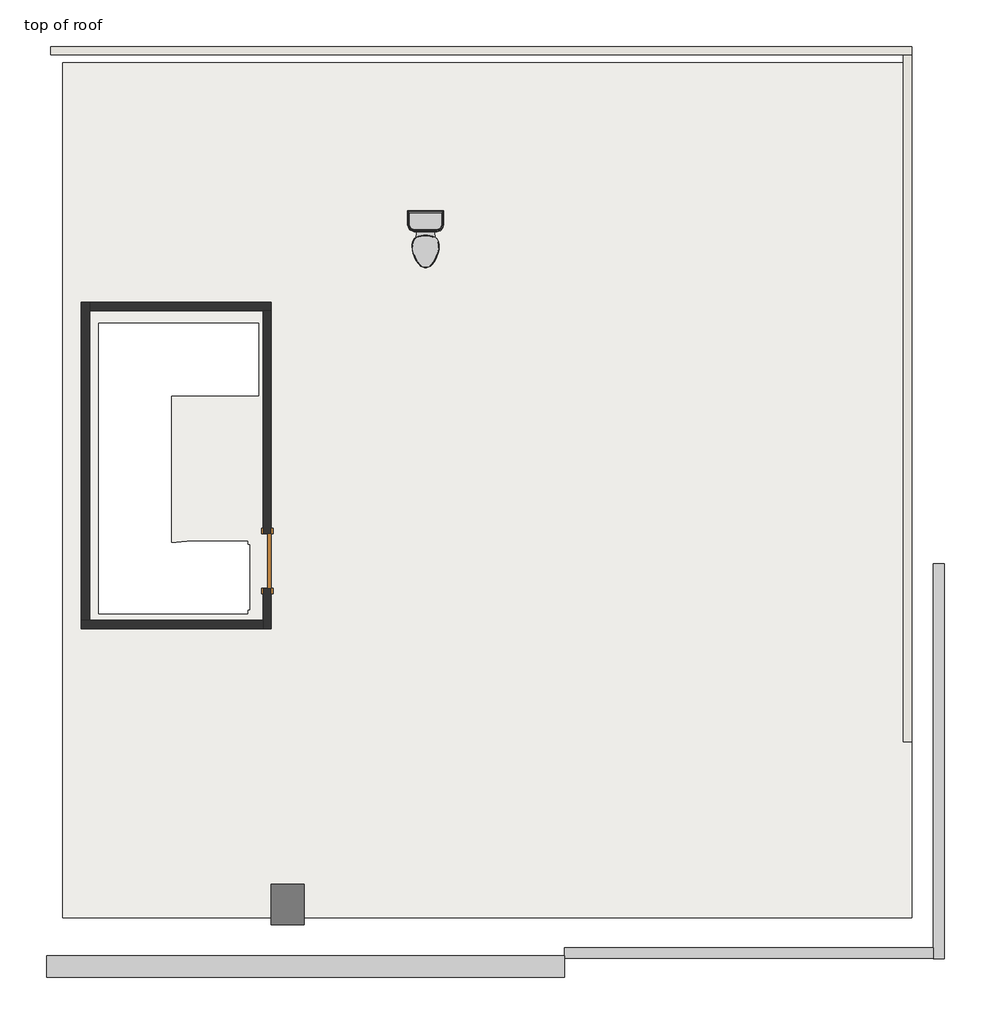
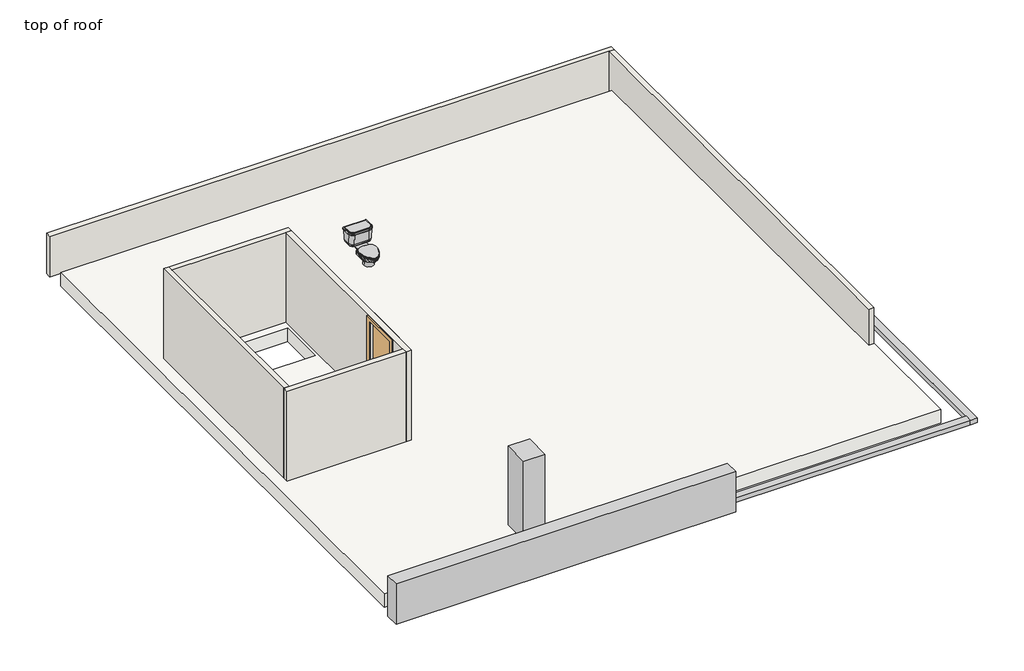
# One storey, incomplete: 6 walls, 4 proxies, 1 door, 1 flow terminal, 1 slab.
"""IFC4 building model written with IfcOpenShell, lengths in millimetres."""

from ifc_helpers import new_model, si_unit, frame, origin, place, context, project, spatial, polyline, outline, extrude, faceted_brep, transform, mapped, element, save
from components import generic_models_10_generic_models_10_e252aed2, generic_models_11_generic_models_11_52537d9e, generic_models_2_generic_models_2_cf9e9294, generic_models_22_generic_models_22_43b51bfc, door_f2b275c1, toilet_domestic_3d_toilet_domestic_3d_ba6479b0, toilet_domestic_3d_toilet_domestic_3d_30431060

model = new_model("IFC4")

# Units and contexts
model_context = context("Model", 3, world=origin())
ifc_project = project(units=[si_unit("LENGTHUNIT", "METRE", prefix="MILLI")], contexts=[model_context])

# Site, building, storey
site = spatial("IfcSite", under=ifc_project)
building = spatial("IfcBuilding", under=site)
storey = spatial("IfcBuildingStorey", under=building, Name="top of roof", Elevation=6400.8)

# Proxies
placement = place(None, origin())
generic_models_10_generic_models_10_shape = generic_models_10_generic_models_10_e252aed2(model_context)
element("IfcBuildingElementProxy", 1, Name="Generic Models 10 : Generic Models 10", ObjectType="Generic Models 10 : Generic Models 10", at=placement, inside=storey, context=model_context, shape_type="MappedRepresentation", body=[
    mapped(generic_models_10_generic_models_10_shape, transform((0.0, 0.0, 0.0), x_axis=(1.0, 0.0, 0.0), y_axis=(0.0, 1.0, 0.0), z_axis=(0.0, 0.0, 1.0))),
])
generic_models_11_generic_models_11_shape = generic_models_11_generic_models_11_52537d9e(model_context)
element("IfcBuildingElementProxy", 2, Name="Generic Models 11 : Generic Models 11", ObjectType="Generic Models 11 : Generic Models 11", at=placement, inside=storey, context=model_context, shape_type="MappedRepresentation", body=[
    mapped(generic_models_11_generic_models_11_shape, transform((0.0, 0.0, 0.0), x_axis=(1.0, 0.0, 0.0), y_axis=(0.0, 1.0, 0.0), z_axis=(0.0, 0.0, 1.0))),
])
generic_models_2_generic_models_2_shape = generic_models_2_generic_models_2_cf9e9294(model_context)
element("IfcBuildingElementProxy", 3, Name="Generic Models 2 : Generic Models 2", ObjectType="Generic Models 2 : Generic Models 2", at=placement, inside=storey, context=model_context, shape_type="MappedRepresentation", body=[
    mapped(generic_models_2_generic_models_2_shape, transform((0.0, 0.0, 0.0), x_axis=(1.0, 0.0, 0.0), y_axis=(0.0, 1.0, 0.0), z_axis=(0.0, 0.0, 1.0))),
])
generic_models_22_generic_models_22_shape = generic_models_22_generic_models_22_43b51bfc(model_context)
element("IfcBuildingElementProxy", 4, Name="Generic Models 22 : Generic Models 22", ObjectType="Generic Models 22 : Generic Models 22", at=placement, inside=storey, context=model_context, shape_type="MappedRepresentation", body=[
    mapped(generic_models_22_generic_models_22_shape, transform((0.0, 1066.8, 0.0), x_axis=(1.0, 0.0, 0.0), y_axis=(0.0, 1.0, 0.0), z_axis=(0.0, 0.0, 1.0))),
])

# Door
door_shape = door_f2b275c1(model_context)
element("IfcDoor", 5, ObjectType="Single-Flush : 30\" x 80\"", at=placement, inside=storey, context=model_context, shape_type="MappedRepresentation", body=[
    mapped(door_shape, transform((-8958.2763881, -2229.5563549, 6400.8), x_axis=(0.0, 1.0, 0.0), y_axis=(-1.0, 0.0, 0.0), z_axis=(0.0, 0.0, 1.0))),
])

# Flow terminal
toilet_domestic_3d_toilet_domestic_3d_shape = toilet_domestic_3d_toilet_domestic_3d_ba6479b0(model_context)
toilet_domestic_3d_toilet_domestic_3d_2_shape = toilet_domestic_3d_toilet_domestic_3d_30431060(model_context)
element("IfcFlowTerminal", 6, ObjectType="Toilet-Domestic-3D : Toilet-Domestic-3D", at=placement, inside=storey, context=model_context, shape_type="MappedRepresentation", body=[
    mapped(toilet_domestic_3d_toilet_domestic_3d_shape, transform((-6741.0586008, 2177.219561, 6400.8), x_axis=(1.0, 0.0, 0.0), y_axis=(0.0, 1.0, 0.0), z_axis=(0.0, 0.0, 1.0))),
    mapped(toilet_domestic_3d_toilet_domestic_3d_2_shape, transform((-6741.0586008, 2177.219561, 6400.8), x_axis=(1.0, 0.0, 0.0), y_axis=(0.0, 1.0, 0.0), z_axis=(0.0, 0.0, 1.0))),
])

# Slab
element("IfcSlab", 7, ObjectType="ROOFING 6\"", at=placement, inside=storey, context=model_context, shape_type="SweptSolid", body=[
    extrude(outline(polyline([(66.1413992, 4742.0155883), (66.1413992, -7221.3844117), (-11821.0586008, -7221.3844117), (-11821.0586008, 4742.0155883), (66.1413992, 4742.0155883)]), holes=[polyline([(-9079.7156858, 1095.9115003), (-11318.9522729, 1095.9115003), (-11318.9522729, -2966.8844117), (-9236.1522729, -2966.8844117), (-9236.1522729, -2916.0844117), (-9204.4022729, -2916.0844117), (-9204.4022729, -2001.6844117), (-9236.1522729, -2001.6844117), (-9236.1522729, -1950.8844117), (-10077.172189, -1950.8844117), (-10302.9522729, -1976.0280655), (-10302.9522729, 79.9115003), (-9079.7156858, 79.9115003), (-9079.7156858, 1095.9115003)])]), frame((0.0, 0.0, 6197.6), z_axis=(0.0, 0.0, 1.0), x_axis=(1.0, 0.0, 0.0)), (0.0, 0.0, 1.0), 304.8),
])

# Walls
element("IfcWall", 8, at=placement, inside=storey, context=model_context, shape_type="Brep", body=[
    faceted_brep([(-11992.5086008, 4856.3155883, 6400.8), (-48.1586008, 4856.3155883, 6400.8), (66.1413992, 4856.3155883, 6400.8), (66.1413992, 4856.3155883, 7315.2), (-48.1586008, 4856.3155883, 7315.2), (-11992.5086008, 4856.3155883, 7315.2), (-11992.5086008, 4970.6155883, 6400.8), (-11992.5086008, 4970.6155883, 7315.2), (66.1413992, 4970.6155883, 7315.2), (66.1413992, 4970.6155883, 6400.8)], [[[0, 1, 2, 3, 4, 5]], [[6, 7, 8, 9]], [[2, 1, 0, 6, 9]], [[5, 4, 3, 8, 7]], [[0, 5, 7, 6]], [[3, 2, 9, 8]]]),
])
element("IfcWall", 9, at=placement, inside=storey, context=model_context, shape_type="SweptSolid", body=[
    extrude(outline(polyline([(-48.1586008, -4757.5844117), (-48.1586008, 4856.3155883), (66.1413992, 4856.3155883), (66.1413992, -4757.5844117), (-48.1586008, -4757.5844117)])), frame((0.0, 0.0, 6400.8), z_axis=(0.0, 0.0, 1.0), x_axis=(1.0, 0.0, 0.0)), (0.0, 0.0, 1.0), 914.4),
])
element("IfcWall", 10, at=placement, inside=storey, context=model_context, shape_type="Brep", body=[
    faceted_brep([(-11561.5206309, -3175.7063549, 6400.8), (-9015.4263881, -3175.7063549, 6400.8), (-9015.4263881, -3175.7063549, 8534.4), (-11561.5206309, -3175.7063549, 8534.4), (-11561.5206309, -3061.4063549, 6400.8), (-11561.5206309, -3061.4063549, 8534.4), (-11447.2206309, -3061.4063549, 8534.4), (-9015.4263881, -3061.4063549, 8534.4), (-9015.4263881, -3061.4063549, 6400.8), (-11447.2206309, -3061.4063549, 6400.8)], [[[0, 1, 2, 3]], [[4, 5, 6, 7, 8, 9]], [[1, 0, 4, 9, 8]], [[3, 2, 7, 6, 5]], [[0, 3, 5, 4]], [[2, 1, 8, 7]]]),
])
element("IfcWall", 11, at=placement, inside=storey, context=model_context, shape_type="Brep", body=[
    faceted_brep([(-11561.5206309, 1389.2155883, 6400.8), (-11561.5206309, -3061.4063549, 6400.8), (-11561.5206309, -3061.4063549, 8534.4), (-11561.5206309, 1389.2155883, 8534.4), (-11447.2206309, 1389.2155883, 6400.8), (-11447.2206309, 1389.2155883, 8534.4), (-11447.2206309, 1274.9155883, 8534.4), (-11447.2206309, -3061.4063549, 8534.4), (-11447.2206309, -3061.4063549, 6400.8), (-11447.2206309, 1274.9155883, 6400.8)], [[[0, 1, 2, 3]], [[4, 5, 6, 7, 8, 9]], [[1, 0, 4, 9, 8]], [[3, 2, 7, 6, 5]], [[0, 3, 5, 4]], [[2, 1, 8, 7]]]),
])
element("IfcWall", 12, at=placement, inside=storey, context=model_context, shape_type="Brep", body=[
    faceted_brep([(-8901.1263881, 1389.2155883, 6400.8), (-11447.2206309, 1389.2155883, 6400.8), (-11447.2206309, 1389.2155883, 8534.4), (-8901.1263881, 1389.2155883, 8534.4), (-8901.1263881, 1274.9155883, 6400.8), (-8901.1263881, 1274.9155883, 8534.4), (-9015.4263881, 1274.9155883, 8534.4), (-11447.2206309, 1274.9155883, 8534.4), (-11447.2206309, 1274.9155883, 6400.8), (-9015.4263881, 1274.9155883, 6400.8)], [[[0, 1, 2, 3]], [[4, 5, 6, 7, 8, 9]], [[1, 0, 4, 9, 8]], [[3, 2, 7, 6, 5]], [[0, 3, 5, 4]], [[2, 1, 8, 7]]]),
])
element("IfcWall", 13, at=placement, inside=storey, context=model_context, shape_type="Brep", body=[
    faceted_brep([(-8901.1263881, -1848.5563549, 8432.8), (-8901.1263881, -1848.5563549, 6400.8), (-8901.1263881, 1274.9155883, 6400.8), (-8901.1263881, 1274.9155883, 8534.4), (-8901.1263881, -3175.7063549, 8534.4), (-8901.1263881, -3175.7063549, 6400.8), (-8901.1263881, -2610.5563549, 6400.8), (-8901.1263881, -2610.5563549, 8432.8), (-9015.4263881, 1274.9155883, 6400.8), (-9015.4263881, -1848.5563549, 6400.8), (-9015.4263881, -1848.5563549, 8432.8), (-9015.4263881, -2610.5563549, 8432.8), (-9015.4263881, -2610.5563549, 6400.8), (-9015.4263881, -3061.4063549, 6400.8), (-9015.4263881, -3175.7063549, 6400.8), (-9015.4263881, -3175.7063549, 8534.4), (-9015.4263881, -3061.4063549, 8534.4), (-9015.4263881, 1274.9155883, 8534.4)], [[[0, 1, 2, 3, 4, 5, 6, 7]], [[8, 9, 10, 11, 12, 13, 14, 15, 16, 17]], [[6, 5, 14, 13, 12]], [[2, 1, 9, 8]], [[4, 3, 17, 16, 15]], [[5, 4, 15, 14]], [[3, 2, 8, 17]], [[10, 9, 1, 0]], [[11, 10, 0, 7]], [[12, 11, 7, 6]]]),
])

save(model, "model.ifc")

# Revit data of these elements
# Type "Single-Flush : 30\" x 80\""
#   Type Mark = "5"
#   Construction Type Id = "MDOOR"
#   Assembly Code = "C1020"
#   Analytic Construction = "Metal"
#   Thickness = 0' - 2"
#   Heat Transfer Coefficient (U) = 0.651978 BTU/(h·ft²·°F)
#   Height = 6' - 8"
#   Trim Projection Ext = 0' - 1"
#   Trim Projection Int = 0' - 1"
#   Trim Width = 0' - 3"
#   Width = 2' - 6"
#   Define Thermal Properties by = 1
#   Define Thermal Properties by = 1
#   Door Material = Door - Panel
#   Frame Material = Door - Frame
#   Visual Light Transmittance = 0
#   Solar Heat Gain Coefficient = 0
#   Function = (empty or 0)
#   Wall Closure = (empty or 0)
# Type "Toilet-Domestic-3D : Toilet-Domestic-3D"
#   Assembly Code = "D2010110"
#   Toilet - Bowl/Basin Material = Porcelain, Linen
#   Toilet - Seat Material = Laminate, Linen, Matte
#   Default Elevation = 0
# Type "ROOFING 6\""
#   Assembly Code = "B1010"
#   Function = 0
#   Layers, outside or top first: 1' - 0" "ROOFING MATERIAL 1'" (function 1)
# Type
#   Assembly Code = "B2010"
#   Layers, outside or top first: 0' - 4 1/2" "OFF WHITE COLOUR" (function 1)
# Element 1 (IfcBuildingElementProxy, "Generic Models 10 : Generic Models 10")
#   Phase Created = New Construction
#   Materials on its faces: "Clad - White"
# Element 2 (IfcBuildingElementProxy, "Generic Models 11 : Generic Models 11")
#   Phase Created = New Construction
#   Materials on its faces: "Clad - White"
# Element 3 (IfcBuildingElementProxy, "Generic Models 2 : Generic Models 2")
#   Phase Created = New Construction
#   Materials on its faces: "ESPRESSO"
# Element 4 (IfcBuildingElementProxy, "Generic Models 22 : Generic Models 22")
#   Phase Created = New Construction
#   Materials on its faces: "ESPRESSO"
# Element 5 (IfcDoor, "Single-Flush : 30\" x 80\"")
#   Phase Created = New Construction
#   Materials on its faces: "Door - Frame", "Door - Panel"
# Element 6 (IfcFlowTerminal, "Toilet-Domestic-3D : Toilet-Domestic-3D")
#   Mark = "2"
#   Phase Created = New Construction
#   Materials on its faces: "Porcelain, Linen", "Laminate, Linen, Matte"
# Element 7 (IfcSlab, "ROOFING 6\"")
#   Height Offset From Level = 0' - 4"
#   Phase Created = New Construction
#   Materials on its faces: "ROOFING MATERIAL 1'"
# Elements 8, 9 (IfcWall)
#   Top Offset = 0' - 0"
#   Base Offset = 0' - 0"
#   Unconnected Height = 3' - 0"
#   wall height = 3' - 0"
#   Phase Created = New Construction
#   Base Constraint = top of roof
#   Materials on its faces: "OFF WHITE COLOUR"
# Elements 10, 11, 12, 13 (IfcWall)
#   Top Offset = 0' - 0"
#   Base Offset = 0' - 0"
#   Unconnected Height = 7' - 0"
#   wall height = 7' - 0"
#   Phase Created = New Construction
#   Base Constraint = top of roof
#   Materials on its faces: "OFF WHITE COLOUR"
# Materials
#   "Door - Panel": class "Wood", colour RGB 210 159 95, transparency 0, Cost = 0
#   "Door - Frame": colour RGB 118 70 51, transparency 0, Cost = 0
#   "Porcelain, Linen": class "Ceramic", colour RGB 249 239 230, transparency 0, Description = "Porcelain, linen", Cost = 0
#   "Laminate, Linen, Matte": class "Plastic", colour RGB 249 239 230, transparency 0, Description = "Plastic Laminate - Linen, Matte", Cost = 0
#   "ROOFING MATERIAL 1'": class "Generic", colour RGB 120 120 120, transparency 0, Cost = 0
#   "OFF WHITE COLOUR": class "Generic", colour RGB 120 120 120, transparency 0, Cost = 0
#   "Clad - White": class "Wood", colour RGB 242 242 238, transparency 0, Cost = 0
#   "ESPRESSO": class "Generic", colour RGB 120 120 120, transparency 0, Cost = 0
